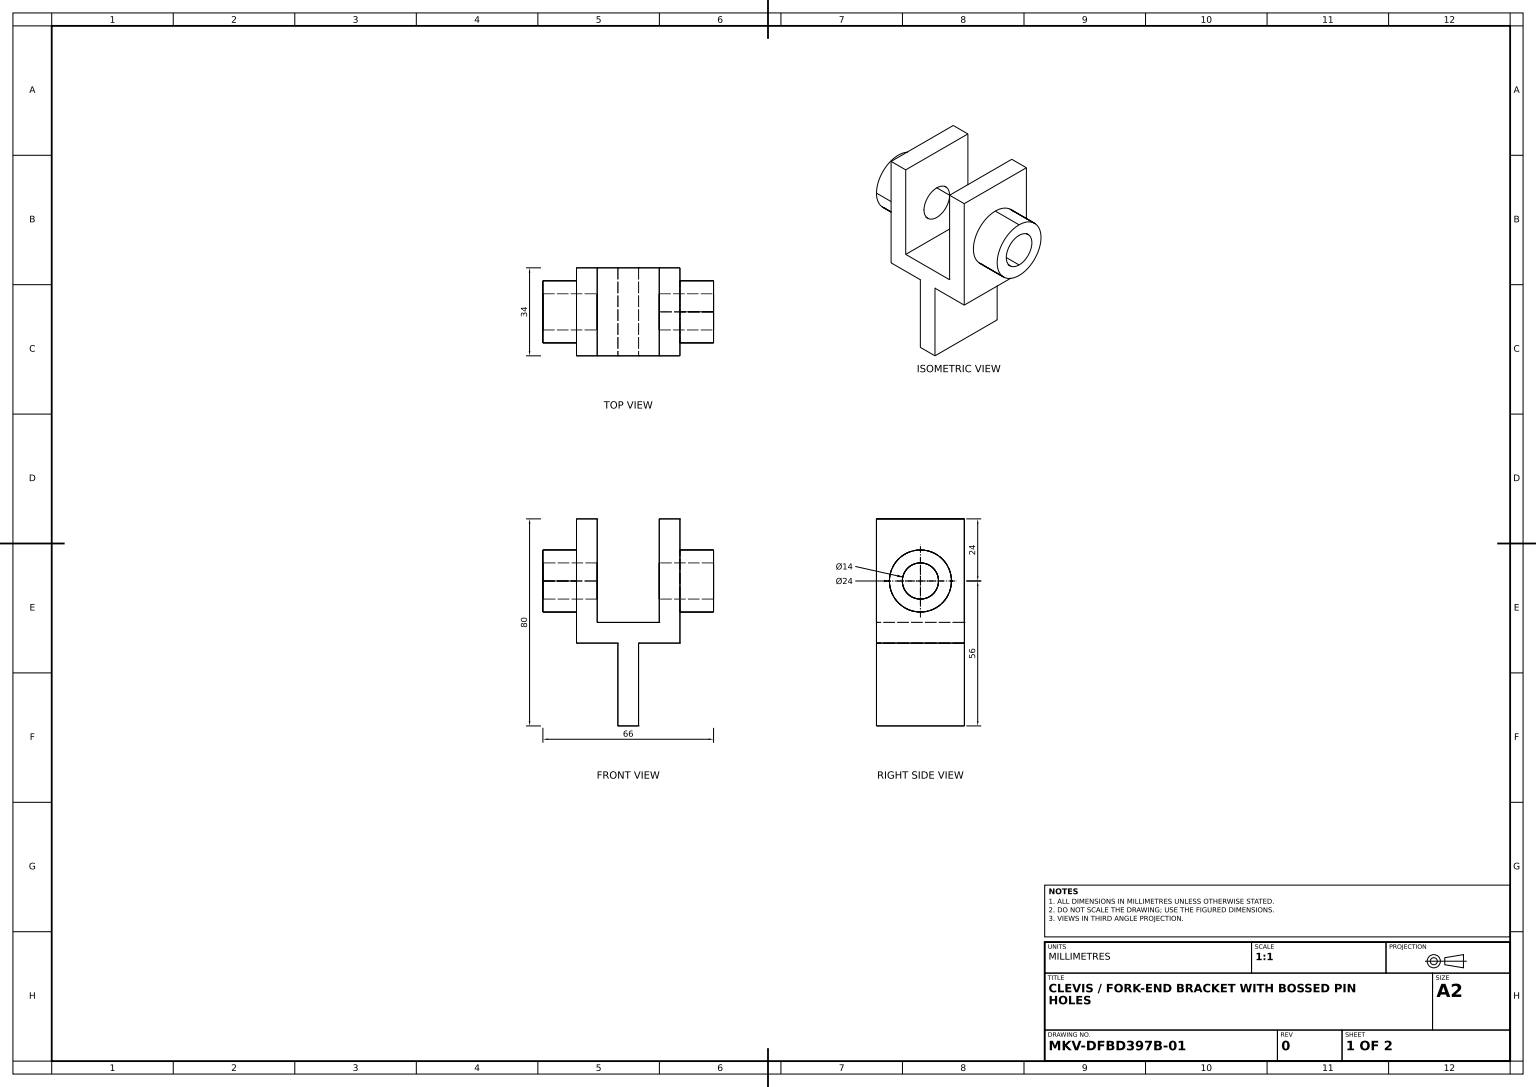
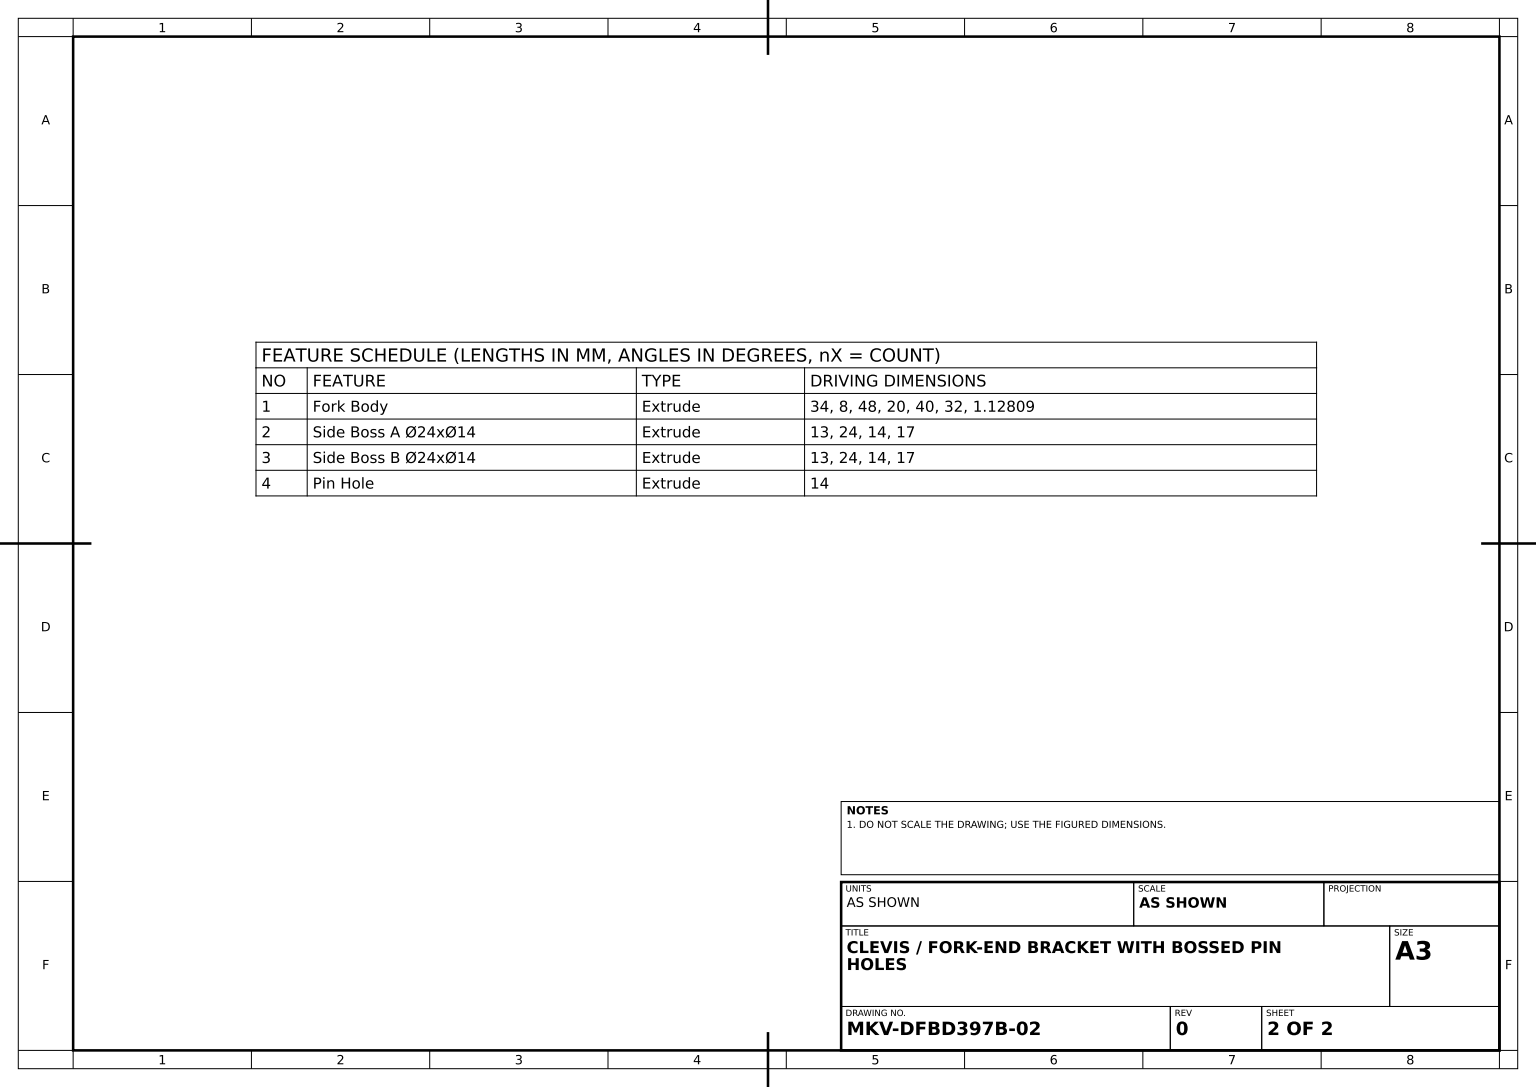
SolidWorks part; units mm, degrees
material "Plain Carbon Steel"
ref_plane "Front Plane" through (0, 0, 0) normal (0, 0, 1) x (1, 0, 0)
ref_plane "Top Plane" through (0, 0, 0) normal (0, 1, 0) x (1, 0, 0)
ref_plane "Right Plane" through (0, 0, 0) normal (1, 0, 0) x (0, 0, -1)
sketch "Fork Profile Sketch" plane through (0, 0, 0) normal (0, 0, 1) x (1, 0, 0)
  line L1 (-2.8719, 0) -> (-2.8719, 32)
  line L2 (-2.8719, 32) -> (-18.8719, 32)
  line L3 (-18.8719, 32) -> (-18.8719, 80)
  line L4 (-18.8719, 80) -> (-10.8719, 80)
  line L5 (-10.8719, 80) -> (-10.8719, 40)
  line L6 (-10.8719, 40) -> (13.1281, 40)
  line L7 (13.1281, 40) -> (13.1281, 80)
  line L8 (13.1281, 80) -> (21.1281, 80)
  line L9 (21.1281, 80) -> (21.1281, 32)
  line L10 (21.1281, 32) -> (5.1281, 32)
  line L11 (5.1281, 32) -> (5.1281, 0)
  line L13 (-2.8719, 0) -> (5.1281, 0)
  point P0 (1.1281, 0)
  dimension "D1" = 8
  dimension "D2" = 20
  dimension "D3" = 40
  dimension "D4" = 48
  dimension "D5" = 8
  dimension "D6" = 8
  dimension "D7" = 8
  dimension "D8" = 32
  dimension "D9" = 1.1281
extrude "Fork Body" add sketch "Fork Profile Sketch" against normal blind 34
sketch "Side Boss A Sketch" plane through (21.1281, 0, 0) normal (1, 0, 0) x (0, 0, -1)
  line L0 (34, 32) -> (0, 32) construction
  line L1 (34, 32) -> (34, 80) construction
  circle A0 centre (17, 56) radius 12
  circle A1 centre (17, 56) radius 7
  dimension "D1" = 24
  dimension "D2" = 14
  dimension "D3" = 24
  dimension "D4" = 17
extrude "Side Boss A Ø24xØ14" add sketch "Side Boss A Sketch" along normal blind 13
sketch "Side Boss B Sketch" plane through (-18.8719, 0, 0) normal (-1, 0, 0) x (0, 0, 1)
  line L0 (-34, 32) -> (0, 32) construction
  line L1 (-34, 80) -> (-34, 32) construction
  circle A0 centre (-17, 56) radius 12
  circle A1 centre (-17, 56) radius 7
  dimension "D1" = 24
  dimension "D2" = 14
  dimension "D3" = 24
  dimension "D4" = 17
extrude "Side Boss B Ø24xØ14" add sketch "Side Boss B Sketch" along normal blind 13
sketch "Pin Hole Sketch" plane through (-18.8719, 0, 0) normal (-1, 0, 0) x (0, 0, 1)
  circle A0 centre (-17, 56) radius 7
  dimension "D1" = 14
extrude "Pin Hole" cut sketch "Pin Hole Sketch" against normal through all
